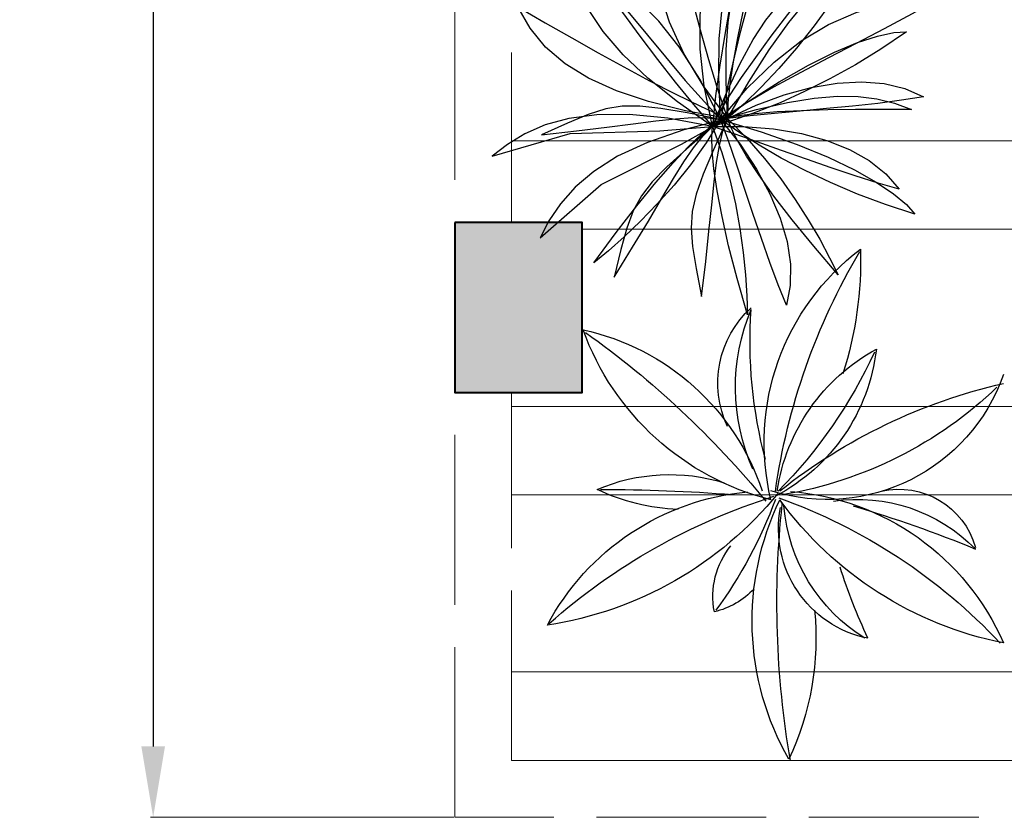
# Model space of a CAD drawing. Units: inches. Extents: x 351 to 1738, y -265 to 286.
# Tile 8 of 38: x 1004 to 1074, y -203 to -147. Entities that reach past the tile are written whole.
import ezdxf

# ---------------------------------------------------------------- set-up
doc = ezdxf.new("R2010")
doc.units = ezdxf.units.IN
doc.header["$MEASUREMENT"] = 0
doc.linetypes.add('ACAD_ISO02W100', pattern=[15, 12, -3])
for name, color, linetype, lineweight in [('A-ANNO-DIMS', 2, 'Continuous', 18), ('A-COLS', 7, 'Continuous', 40), ('A-COLS-PATT', 6, 'Continuous', 13), ('A-FLOR-OVHD', 1, 'ACAD_ISO02W100', 18), ('A-FLOR-PATT', 9, 'Continuous', 9), ('A-WALL', 7, 'Continuous', 35)]:
    doc.layers.add(name, color=color, linetype=linetype, lineweight=lineweight)
for name, color, linetype in [('CAY', 94, 'Continuous'), ('CHITIET', 144, 'Continuous'), ('DIENHOA', 3, 'Continuous'), ('netmanh', 9, 'Continuous'), ('VATDUNG', 9, 'Continuous')]:
    doc.layers.add(name, color=color, linetype=linetype)
doc.styles.get("Standard").update_dxf_attribs({"font": 'arial.ttf'})
doc.dimstyles.get("Standard").update_dxf_attribs({"dimtxt": 8, "dimasz": 5, "dimexe": 0.18, "dimexo": 0.0625, "dimgap": 0.09, "dimtad": 1, "dimtoh": 1, "dimzin": 0, "dimdsep": 46, "dimlunit": 4, "dimtxsty": 'Standard', "dimcen": 0, "dimclre": 256, "dimadec": 0, "dimazin": 0, "dimtfac": 1, "dimtofl": 0, "dimtmove": 0, "dimatfit": 3, "dimfxl": 1, "dimtolj": 1, "dimtzin": 0, "dimlwe": -1, "dimarcsym": 0})

# ---------------------------------------------------------------- blocks, each defined once
blk = doc.blocks.new('*D8')
at = {"layer": 'A-ANNO-DIMS', "color": 0, "transparency": 16777216}
for p, q in [((1034.642, 255.963), (1013.221, 255.963)), ((1034.642, -203.037), (1013.221, -203.037))]:
    blk.add_line(p, q, dxfattribs=at)
at = {"layer": 'A-ANNO-DIMS', "color": 0, "lineweight": -2, "transparency": 16777216}
blk.add_line((1013.401, 250.963), (1013.401, -198.037), dxfattribs=at)
at = {"layer": 'A-ANNO-DIMS', "color": 0, "transparency": 16777216}
for points in [[(1012.568, 250.963), (1014.235, 250.963), (1013.401, 255.963)], [(1012.568, -198.037), (1014.235, -198.037), (1013.401, -203.037)]]:
    blk.add_solid(points, dxfattribs=at)
at = {"layer": 'Defpoints', "color": 0, "transparency": 16777216}
for p in [(1034.704, 255.963), (1013.401, -203.037), (1034.704, -203.037)]:
    blk.add_point(p, dxfattribs=at)
at = {"layer": 'A-ANNO-DIMS', "color": 0, "transparency": 16777216, "insert": (1009.224, 26.463), "char_height": 8, "attachment_point": 5, "rotation": 90}
blk.add_mtext('\\A1;38\'-3"', dxfattribs=at)
blk = doc.blocks.new('A$C5431134F')
at = {"layer": 'VATDUNG'}
for centre, radius, start, end in [((2160.8, 1662), 1245, 150.2411, 205.809), ((5177, 1582.5), 4150.3, 170.24, 186.1148), ((-65.9, 1738.8), 1267.2, 354.3326, 25.2804), ((1532.8, 1250.1), 499, 101.4267, 190.9877), ((193.1, 3473.3), 2507.8, 289.6318, 316.9416), ((2357.8, 162.2), 1629.1, 101.2486, 143.9899), ((1828.1, 1082.8), 773.2, 121.9055, 175.1859), ((1000.7, 2213.1), 1133.8, 274.4073, 336.4431), ((3715.1, 660.2), 2523.5, 154.6853, 162.4501), ((-246.7, 51.1), 1647.5, 39.15, 81.389), ((1000.7, 2213.1), 1133.8, 208.0484, 264.6491), ((1859.5, 3770.4), 2797.6, 228.5745, 252.3842), ((1101.5, 1552.5), 361.2, 169.1166, 218.9556), ((667.9, 1279.8), 349.9, 42.8374, 76.9786), ((-929.9, 388.9), 2082.1, 20.5138, 36.0242), ((1386.4, 1856.4), 738.5, 261.6389, 315.6255), ((-169.9, 6392.7), 5465.7, 286.3355, 292.415), ((1571.2, 1428.8), 356.3, 257.3557, 344.3532), ((624.5, 223.6), 940.4, 92.4374, 115.2956), ((1294.4, -49.6), 1206.1, 104.1284, 160.1468), ((-2233.8, 3749.8), 4146.2, 305.4464, 320.7382), ((2052.7, 864.5), 1083.3, 166.3603, 232.9474), ((1250.8, 281.5), 836.9, 19.4342, 107.4357), ((625, 349.3), 851.8, 6.5073, 62.3609), ((-65.9, 1738.8), 1267.2, 330.7697, 331.9367), ((-70, 1420), 1084.7, 282.2423, 341.7321), ((546.4, 1826.6), 819.5, 246.7315, 287.3971), ((248.9, 8461.8), 7388, 269.91003, 274.50199), ((3885.3, 1488.7), 2894, 188.0959, 210.7226), ((1889.6, 1210.8), 871.9, 188.5552, 241.3289), ((-527.8, -458.7), 2192.5, 24.7599, 44.6473), ((2594.9, 3037.7), 2500, 231.5416, 257.1764), ((754.1, -691.9), 1814.1, 46.1483, 80.3711), ((1738.9, 617.5), 897.6, 155.9893, 202.84), ((2946.5, 414), 2039.9, 165.0604, 184.0737), ((1214.1, 597.8), 452.1, 154.5276, 228.0163), ((-246.7, 51.1), 1647.5, 358.2222, 17.8583)]:
    blk.add_arc(centre, radius, start, end, dxfattribs=at)
blk = doc.blocks.new('A$C5A8625A6')
at = {"layer": 'CHITIET', "ltscale": 50, "xscale": -0.49, "yscale": 0.49, "zscale": 0.49, "rotation": 180}
blk.add_blockref('A$C5431134F', (0, 1120.2), dxfattribs=at)
blk = doc.blocks.new('A$C18571848')
at = {"layer": 'netmanh', "xscale": 0.5393606399999998, "yscale": 0.5393606399999998, "zscale": 0.5393606399999998}
blk.add_blockref('A$C5A8625A6', (0, 0), dxfattribs=at)
blk = doc.blocks.new('Cay03_mb')
at = {"layer": 'DIENHOA'}
for p, q in [((118.6, 555.3), (166.2, 599.1)), ((166.2, 599.1), (142.2, 519.4)), ((79.5, 503.7), (118.6, 555.3)), ((48.6, 443.6), (79.5, 503.7)), ((142.2, 519.4), (119, 441.7)), ((25.5, 374.3), (48.6, 443.6)), ((119, 441.7), (96.7, 365.6)), ((-365.2, 390.3), (-414.4, 402.8)), ((-414.4, 402.8), (-240.2, 277.8)), ((-314.9, 371.3), (-365.2, 390.3)), ((-263.5, 343.5), (-314.9, 371.3)), ((9.9, 295.3), (25.5, 374.3)), ((96.7, 365.6), (75.6, 290.6)), ((-211.2, 304.6), (-263.5, 343.5)), ((511, 309.6), (585.9, 313.5)), ((585.9, 313.5), (511.8, 271.4)), ((-158, 252.3), (-211.2, 304.6)), ((1.6, 205.7), (9.9, 295.3)), ((75.6, 290.6), (55.7, 216.3)), ((363.4, 275.4), (436.8, 297.2)), ((436.8, 297.2), (511, 309.6)), ((-240.2, 277.8), (-88.4, 94.9)), ((290.6, 243.2), (363.4, 275.4)), ((511.8, 271.4), (437.6, 231.5)), ((-104.2, 184.4), (-158, 252.3)), ((218.5, 199.8), (290.6, 243.2)), ((55.7, 216.3), (37.3, 142.1)), ((437.6, 231.5), (363.7, 192.9)), ((-49.6, 98.5), (-104.2, 184.4)), ((0.2, 104.9), (1.6, 205.7)), ((147, 144.1), (218.5, 199.8)), ((363.7, 192.9), (290.2, 154.9)), ((37.3, 142.1), (20.5, 67.6)), ((75.9, 75.2), (147, 144.1)), ((290.2, 154.9), (217.4, 116.6)), ((5.4, -7.8), (0.2, 104.9)), ((217.4, 116.6), (145.5, 77.3)), ((-88.4, 94.9), (5.4, -7.8)), ((5.4, -7.8), (-49.6, 98.5)), ((5.4, -7.8), (75.9, 75.2)), ((20.5, 67.6), (5.4, -7.8)), ((145.5, 77.3), (74.7, 36.1)), ((253, 48.9), (314.6, 54.1)), ((314.6, 54.1), (369.2, 53.3)), ((369.2, 53.3), (418.6, 46.8)), ((-254.7, 27.4), (-298.6, 20.1)), ((-208, 27.8), (-254.7, 27.4)), ((-152.7, 21.7), (-208, 27.8)), ((74.7, 36.1), (5.4, -7.8)), ((100.3, 18.4), (182.2, 37.2)), ((182.2, 37.2), (253, 48.9)), ((418.6, 46.8), (464.9, 35.2)), ((464.9, 35.2), (510, 19)), ((-345, 5.4), (-399.6, -17.1)), ((-298.6, 20.1), (-345, 5.4)), ((-83.4, 9.7), (-152.7, 21.7)), ((5.4, -7.8), (-83.4, 9.7)), ((5.4, -7.8), (100.3, 18.4)), ((46.3, 0.9), (5.4, -7.8)), ((96.7, 7.5), (46.3, 0.9)), ((155, 12.2), (96.7, 7.5)), ((219.6, 15.4), (155, 12.2)), ((289, 17.4), (219.6, 15.4)), ((361.6, 18.5), (289, 17.4)), ((435.8, 18.9), (361.6, 18.5)), ((510, 19), (435.8, 18.9)), ((-399.6, -17.1), (-468, -47.9)), ((-295.3, -27.9), (-225.8, -18.9)), ((-225.8, -18.9), (-165.8, -11.3)), ((-165.8, -11.3), (-114, -5.7)), ((-114, -5.7), (-69, -2.9)), ((-69, -2.9), (-29.6, -3.4)), ((-45.1, -46.3), (-16.5, -22.4)), ((5.4, -7.8), (-33.2, -69.5)), ((-29.6, -3.4), (5.4, -7.8)), ((-16.5, -22.4), (5.4, -7.8)), ((5.4, -7.8), (56.8, -73.3)), ((25.9, -64.4), (5.4, -7.8)), ((5.4, -7.8), (112.8, -40.3)), ((53.5, -41.6), (5.4, -7.8)), ((-468, -47.9), (-375.6, -37.8)), ((-375.6, -37.8), (-295.3, -27.9)), ((-79.8, -79.6), (-45.1, -46.3)), ((107, -75.7), (53.5, -41.6)), ((112.8, -40.3), (207.5, -73.8)), ((-33.2, -69.5), (-74.6, -127.3)), ((47, -125.9), (25.9, -64.4)), ((56.8, -73.3), (100.4, -139.1)), ((165.5, -109.6), (107, -75.7)), ((207.5, -73.8), (289.5, -107.6)), ((-120.2, -122.1), (-79.8, -79.6)), ((-165.9, -174.1), (-120.2, -122.1)), ((-74.6, -127.3), (-117.8, -181.1)), ((68.7, -190.6), (47, -125.9)), ((228.7, -142.8), (165.5, -109.6)), ((289.5, -107.6), (359.3, -141.1)), ((100.4, -139.1), (135.9, -204.3)), ((296, -174.7), (228.7, -142.8)), ((359.3, -141.1), (416.9, -173.5)), ((-216.3, -235.6), (-165.9, -174.1)), ((-117.8, -181.1), (-162.1, -230.9)), ((367.1, -204.8), (296, -174.7)), ((416.9, -173.5), (462.6, -204.2)), ((90.8, -256.6), (68.7, -190.6)), ((135.9, -204.3), (162.8, -268.3)), ((441.6, -232.7), (367.1, -204.8)), ((462.6, -204.2), (496.5, -232.5)), ((-162.1, -230.9), (-206.3, -276.5)), ((518.9, -257.7), (441.6, -232.7)), ((496.5, -232.5), (518.9, -257.7)), ((-271, -306.6), (-216.3, -235.6)), ((113.1, -322.2), (90.8, -256.6)), ((-206.3, -276.5), (-249.6, -317.8)), ((162.8, -268.3), (181, -330.4)), ((-329.5, -387.1), (-271, -306.6)), ((-249.6, -317.8), (-291, -354.7)), ((135.4, -385.6), (113.1, -322.2)), ((181, -330.4), (190, -390)), ((-291, -354.7), (-329.5, -387.1)), ((157.6, -445), (135.4, -385.6)), ((190, -390), (189.6, -446.3)), ((179.5, -498.7), (157.6, -445)), ((189.6, -446.3), (179.5, -498.7))]:
    blk.add_line(p, q, dxfattribs=at)
for points in [[(23.7, -5.4), (-41, 82.2), (-91.8, 167.1), (-129.7, 249.5), (-155.6, 329.6), (-170.2, 407.8), (-174.7, 484.2), (-169.8, 559.3), (-156.5, 633.1)], [(-156.5, 633.1), (-132.5, 551.3), (-110.5, 470), (-89.8, 389.2), (-69.6, 309), (-49, 229.4), (-27.1, 150.4), (-3.2, 72.1), (23.7, -5.4)], [(-16.4, -26.7), (-38.3, 80), (-48.9, 178.3), (-48.7, 269), (-38.5, 352.6), (-19.1, 429.7), (9, 501), (44.9, 567.1), (87.9, 628.5)], [(87.9, 628.5), (75.5, 544.2), (61.3, 461.2), (46.1, 379.1), (30.8, 297.8), (16.1, 216.9), (2.9, 136), (-8.3, 54.9), (-16.4, -26.7)], [(-395.6, 473.7), (-347.5, 405.6), (-300.6, 339.5), (-254.3, 275.1), (-208.3, 212.3), (-161.9, 150.9), (-114.8, 90.7), (-66.5, 31.6), (-16.4, -26.7)], [(-16.4, -26.7), (-108.3, 38.6), (-186.9, 101.7), (-252.4, 163.5), (-305.1, 224.4), (-345.4, 285.2), (-373.7, 346.6), (-390.4, 409.2), (-395.6, 473.7)], [(23.7, -5.4), (19.8, 93), (20.3, 177), (25, 248.5), (34, 309.8), (47.3, 362.7), (64.9, 409.3), (86.8, 451.7), (112.9, 491.9)], [(112.9, 491.9), (96, 419.7), (79.5, 347.4), (63.9, 276.5), (50, 208.4), (38.4, 144.8), (29.7, 86.9), (24.6, 36.3), (23.7, -5.4)], [(384.3, 437.5), (342.2, 367.8), (298.1, 301.7), (252.6, 239.4), (206.1, 181.1), (159.4, 127.2), (113, 78), (67.6, 33.6), (23.7, -5.4)], [(23.7, -5.4), (79.9, 91.7), (134.1, 176.2), (185.8, 248.4), (234.3, 308.7), (279, 357.3), (319.3, 394.8), (354.6, 421.4), (384.3, 437.5)], [(273.2, 387.3), (227.6, 328.8), (182.3, 270.1), (138.4, 212.3), (97.2, 156.4), (60, 103.4), (27.8, 54.6), (1.9, 10.8), (-16.4, -26.7)], [(-16.4, -26.7), (21.4, 64.2), (57, 140.3), (91.4, 203.3), (125.2, 255.1), (159.5, 297.5), (195, 332.5), (232.7, 361.8), (273.2, 387.3)], [(-530.5, 289.7), (-458.3, 248.1), (-387.9, 207.8), (-318.9, 168.7), (-250.8, 131.1), (-182.9, 94.8), (-114.9, 59.9), (-46.2, 26.5), (23.7, -5.4)], [(23.7, -5.4), (-87.2, 15.2), (-185, 39.6), (-270.3, 68.2), (-343.7, 101.4), (-405.9, 139.7), (-457.3, 183.5), (-498.7, 233.4), (-530.5, 289.7)], [(496.7, 224), (429.4, 178.4), (361.6, 136.9), (294.1, 99.5), (227.5, 66.1), (162.4, 36.7), (99.7, 11.5), (39.8, -9.7), (-16.4, -26.7)], [(-16.4, -26.7), (75.4, 37.9), (160.1, 91.8), (237.3, 135.7), (306.6, 170), (367.6, 195.4), (419.9, 212.5), (463.1, 221.9), (496.7, 224)], [(23.7, -5.4), (99.3, 29.7), (173.2, 57.1), (244.8, 76.7), (313.3, 88.3), (377.9, 91.8), (437.9, 87), (492.7, 73.8), (541.4, 52)], [(541.4, 52), (484.1, 42.9), (421.2, 34.8), (354.4, 27.6), (285.4, 20.9), (216.1, 14.5), (148.2, 8.1), (83.5, 1.6), (23.7, -5.4)], [(-16.4, -26.7), (-134, -4.7), (-235.3, 5.3), (-322, 4.7), (-395.9, -5), (-458.7, -22.3), (-512.3, -45.7), (-558.2, -73.6), (-598.4, -104.7)], [(-471.9, -320.3), (-310.5, -179.3), (-97.7, -73.3), (23.7, -5.4)], [(23.7, -5.4), (-92.3, -34.8), (-188.4, -68.2), (-266.9, -105.1), (-329.9, -144.9), (-379.7, -187), (-418.5, -230.7), (-448.5, -275.3), (-471.9, -320.3)], [(23.7, -5.4), (-13.6, -87.9), (-41.1, -152.6), (-59.6, -205), (-69.9, -250.7), (-72.8, -295), (-69.2, -343.6), (-59.7, -401.9), (-45.3, -475.5)], [(-45.3, -475.5), (-34.1, -383.2), (-25.4, -302.8), (-18.3, -233.1), (-12, -172.9), (-5.6, -121.2), (2, -76.8), (11.4, -38.5), (23.7, -5.4)], [(316.5, -418.1), (251.4, -342.8), (194.8, -273.3), (146.5, -210.2), (106.3, -153.8), (74.1, -104.7), (49.7, -63.4), (32.9, -30.1), (23.7, -5.4)], [(23.7, -5.4), (74.9, -57.1), (121.8, -110.6), (164.3, -165), (202.7, -219.4), (237, -272.9), (267.3, -324.5), (293.7, -373.2), (316.5, -418.1)], [(-598.4, -104.7), (-392.7, -44.4), (-155, -37.4), (-16.4, -26.7)], [(-276.2, -424.4), (-227.3, -345.4), (-185.7, -276.1), (-150, -215.7), (-119.1, -163.8), (-91.5, -119.5), (-66, -82.3), (-41.4, -51.6), (-16.4, -26.7)], [(-16.4, -26.7), (-84.9, -86), (-137, -133.1), (-175.8, -173), (-204.3, -210), (-225.5, -249.1), (-242.5, -294.7), (-258.4, -351.6), (-276.2, -424.4)], [(76.2, -524.2), (48.8, -428.5), (26.6, -341.7), (9.2, -264.1), (-3.6, -196.1), (-12.3, -138), (-17.1, -90.2), (-18.3, -53), (-16.4, -26.7)], [(-16.4, -26.7), (66.9, -26.6), (145.6, -32.7), (218.8, -44.9), (285.8, -63.1), (345.9, -87.1), (398.4, -116.6), (442.6, -151.6), (477.6, -191.8)], [(477.6, -191.8), (421.8, -176), (361.3, -156.9), (297.6, -135.5), (232.2, -112.6), (166.6, -89.4), (102.3, -66.6), (40.8, -45.4), (-16.4, -26.7)], [(-16.4, -26.7), (8.5, -95.1), (28.5, -163.3), (44.3, -230.6), (56.3, -296.1), (65, -359), (70.9, -418.5), (74.5, -473.9), (76.2, -524.2)]]:
    blk.add_lwpolyline(points, dxfattribs=at)
blk = doc.blocks.new('COL-9x12')
blk.add_lwpolyline([(0, 12), (0, 0), (9, 0), (9, 12)], close=True)

msp = doc.modelspace()

# ---------------------------------------------------------------- hatches: boundary and pattern name
at = {"layer": 'A-COLS-PATT'}
h = msp.add_hatch(color=256, dxfattribs=at)
h.dxf.hatch_style = 1
h.paths.add_polyline_path([(1112.704, 237.963), (1103.704, 237.963), (1103.704, 228.963), (1112.704, 228.963)])
h.paths.add_polyline_path([(1115.704, 237.963), (1112.704, 237.963), (1112.704, 228.963), (1115.704, 228.963)])
h.paths.add_polyline_path([(1043.704, 255.963), (1034.704, 255.963), (1034.704, 243.963), (1043.704, 243.963)])
h.paths.add_polyline_path([(1043.704, 210.963), (1034.704, 210.963), (1034.704, 198.963), (1043.704, 198.963)])
h.paths.add_polyline_path([(1043.704, -45.037), (1034.704, -45.037), (1034.704, -57.037), (1043.704, -57.037)])
h.paths.add_polyline_path([(1112.704, -45.037), (1103.704, -45.037), (1103.704, -57.037), (1112.704, -57.037)])
h.paths.add_polyline_path([(1112.704, -161.037), (1103.704, -161.037), (1103.704, -164.037), (1103.704, -173.037), (1112.704, -173.037)])
h.paths.add_polyline_path([(1043.704, -161.037), (1034.704, -161.037), (1034.704, -173.037), (1043.704, -173.037)])
h.paths.add_polyline_path([(1248.549, -164.037), (1236.549, -164.037), (1236.549, -173.037), (1248.549, -173.037)])
h.paths.add_polyline_path([(1248.549, -50), (1236.549, -50), (1236.549, -59), (1248.549, -59)])
h.paths.add_polyline_path([(1248.704, 73.463), (1244.704, 73.463), (1244.704, 64.463), (1248.704, 64.463)])
h.paths.add_polyline_path([(1244.704, 73.463), (1236.704, 73.463), (1236.704, 64.463), (1244.704, 64.463)])
h.paths.add_polyline_path([(1248.704, 237.963), (1236.704, 237.963), (1236.704, 228.963), (1248.704, 228.963)])
h.paths.add_polyline_path([(1392.204, 237.963), (1380.204, 237.963), (1380.204, 228.963), (1392.204, 228.963)])
h.paths.add_polyline_path([(1536.064, 237.963), (1524.064, 237.963), (1524.064, 228.963), (1536.064, 228.963)])
h.paths.add_polyline_path([(1536.064, 73.463), (1524.064, 73.463), (1524.064, 64.463), (1536.064, 64.463)])
h.paths.add_polyline_path([(1384.204, 73.463), (1380.204, 73.463), (1380.204, 64.463), (1384.204, 64.463)])
h.paths.add_polyline_path([(1392.064, 73.463), (1384.204, 73.463), (1384.204, 64.463), (1392.064, 64.463)])
h.paths.add_polyline_path([(1536.064, -53.037), (1524.064, -53.037), (1524.064, -57.037), (1536.064, -57.037)])
h.paths.add_polyline_path([(1536.064, -48.037), (1524.064, -48.037), (1524.064, -53.037), (1536.064, -53.037)])
h.paths.add_polyline_path([(1392.064, -48.037), (1380.064, -48.037), (1380.064, -56.5), (1380.065, -57.037), (1392.064, -57.037)])
h.paths.add_polyline_path([(1536.064, -164.037), (1524.064, -164.037), (1524.064, -173.037), (1536.064, -173.037)])
at = {"layer": 'A-FLOR-PATT', "transparency": 33554559}
h = msp.add_hatch(dxfattribs=at)
h.set_pattern_fill('ANSI32', color=256, scale=50, angle=135)
h.set_pattern_definition([(180, (1038.704, -199.037), (-2e-15, -18.75), []), (180, (1032.454, -192.787), (-2e-15, -18.75), [])])
h.paths.add_polyline_path([(1248.506, -102.915), (1236.559, -102.916), (1236.553, -56.864), (1112.704, -57.026), (1112.704, -57.037), (1103.704, -57.037), (1103.704, -45.037), (1103.704, 98.963), (1076.434, 98.963), (1076.549, -81.037), (1071.549, -81.037), (1043.704, -81.037), (1038.704, -81.037), (1038.704, -161.037), (1043.704, -161.037), (1043.704, -173.037), (1038.704, -173.037), (1038.704, -199.037), (1562.704, -199.037), (1562.704, -173.037), (1236.549, -173.037), (1236.549, -164.037), (1236.693, -164.037), (1236.676, -150.916), (1248.512, -150.915)])
h.paths.add_polyline_path([(1236.133, -134.078), (1247.348, -134.078), (1247.348, -122.929), (1236.133, -122.929)], flags=24)
h.paths.add_polyline_path([(1308.144, -185.548), (1321.66, -185.548), (1321.66, -174.4), (1308.144, -174.4)], flags=24)
h.paths.add_polyline_path([(1121.632, -122.88), (1179.647, -122.88), (1179.647, -112.309), (1121.632, -112.309)], flags=24)
h.paths.add_polyline_path([(1124.515, -112.593), (1177.986, -112.593), (1177.986, -101.056), (1124.515, -101.056)], flags=24)
h.paths.add_polyline_path([(1091.374, 23.58), (1104.89, 23.58), (1104.89, 34.728), (1091.374, 34.728)], flags=24)

# ---------------------------------------------------------------- linework, layer by layer
at = {"layer": 'A-FLOR-OVHD'}
for p, q in [((1034.704, -203.037), (1034.704, -81.037)), ((1038.704, -161.037), (1038.704, -81.037)), ((1038.704, -199.037), (1038.704, -173.037)), ((1562.704, -199.037), (1038.704, -199.037)), ((1566.704, -203.037), (1034.704, -203.037))]:
    msp.add_line(p, q, dxfattribs=at)
at = {"layer": 'A-WALL'}
msp.add_line((1034.704, -173.037), (1043.704, -173.037), dxfattribs=at)

# ---------------------------------------------------------------- block references
at = {"layer": 'A-COLS'}
msp.add_blockref('COL-9x12', (1034.704, -173.037), dxfattribs=at)
at = {"layer": 'CAY'}
for name, p, xscale, yscale, zscale in [('Cay03_mb', (1053.334, -153.565), 0.0267074520028285, 0.0267074520028285, 0.0267074520028285), ('A$C18571848', (1041.241, -199.037), 0.0597507335965459, 0.0597507335965459, 0.0597507335965459)]:
    msp.add_blockref(name, p, dxfattribs=dict(at, xscale=xscale, yscale=yscale, zscale=zscale))

# ---------------------------------------------------------------- dimensions: what is measured, and where the dimension line sits
at = {"layer": 'A-ANNO-DIMS'}
dim = msp.add_linear_dim(base=(1013.401, -203.037), p1=(1034.704, 255.963), p2=(1034.704, -203.037), angle=90, dimstyle='Standard', override={"dimclrd": 0, "dimclre": 0, "dimclrt": 0}, dxfattribs=at)
dim.commit()
dim.dimension.update_dxf_attribs({"geometry": '*D8', "text_midpoint": (1013.401, 26.463), "dimtype": 160})

doc.saveas('drawing.dxf')
